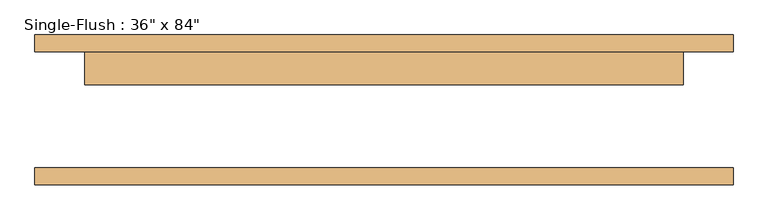
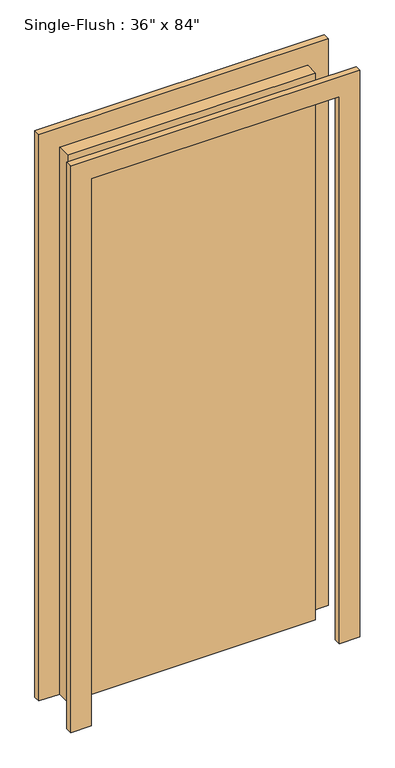
"""IFC4 building model written with IfcOpenShell, lengths in millimetres: door geometry."""

from ifc_helpers import new_model, si_unit, frame, origin, origin_with_axes, place, context, project, spatial, polyline, outline, extrude, source, transform, mapped, element, save


def door_90112511(model_context):
    return source(origin(), model_context, "Body", "SweptSolid", [
        extrude(outline(polyline([(2209.8, -533.4), (0.0, -533.4), (0.0, -457.2), (2133.6, -457.2), (2133.6, 457.2), (0.0, 457.2), (0.0, 533.4), (2209.8, 533.4), (2209.8, -533.4)])), frame((0.0, 88.9, 0.0), z_axis=(0.0, 1.0, 0.0), x_axis=(0.0, 0.0, 1.0)), (0.0, 0.0, 1.0), 25.4),
        extrude(outline(polyline([(2209.8, 533.4), (2209.8, -533.4), (0.0, -533.4), (0.0, -457.2), (2133.6, -457.2), (2133.6, 457.2), (0.0, 457.2), (0.0, 533.4), (2209.8, 533.4)])), frame((0.0, -114.3, 0.0), z_axis=(0.0, 1.0, 0.0), x_axis=(0.0, 0.0, 1.0)), (0.0, 0.0, 1.0), 25.4),
        extrude(outline(polyline([(457.2, 38.1), (-457.2, 38.1), (-457.2, 88.9), (457.2, 88.9), (457.2, 38.1)])), origin_with_axes(), (0.0, 0.0, 1.0), 2133.6),
    ])


if __name__ == "__main__":
    model = new_model("IFC4")
    model_context = context("Model", 3, world=origin())
    ifc_project = project(units=[si_unit("LENGTHUNIT", "METRE", prefix="MILLI")], contexts=[model_context])
    site = spatial("IfcSite", under=ifc_project)
    building = spatial("IfcBuilding", under=site)
    placement = place(None, origin())
    door_shape = door_90112511(model_context)
    element("IfcDoor", 1, ObjectType="Single-Flush : 36\" x 84\"", at=placement, inside=building, context=model_context, shape_type="MappedRepresentation", body=[
        mapped(door_shape, transform((0.0, 0.0, 0.0), x_axis=(1.0, 0.0, 0.0), y_axis=(0.0, 1.0, 0.0), z_axis=(0.0, 0.0, 1.0))),
    ])
    save(model, "model.ifc")

# Revit data of these elements
# Type "Single-Flush : 36\" x 84\""
#   Type Mark = "1"
#   Construction Type Id = "MDOOR"
#   Assembly Code = "C1020"
#   Analytic Construction = "Metal"
#   Thickness = 0' - 2"
#   Heat Transfer Coefficient (U) = 0.651978 BTU/(h·ft²·°F)
#   Height = 7' - 0"
#   Trim Projection Ext = 0' - 1"
#   Trim Projection Int = 0' - 1"
#   Trim Width = 0' - 3"
#   Width = 3' - 0"
#   Define Thermal Properties by = 1
#   Door Material = Door - Panel
#   Frame Material = Door - Frame
#   Visual Light Transmittance = 0
#   Solar Heat Gain Coefficient = 0
#   Function = (empty or 0)
#   Wall Closure = (empty or 0)
# Element 1 (IfcDoor, "Single-Flush : 36\" x 84\"")
#   Materials on its faces: "Door - Frame", "Door - Panel"
# Materials
#   "Door - Panel": class "Wood", colour RGB 210 159 95, transparency 0
#   "Door - Frame": colour RGB 118 70 51, transparency 0
